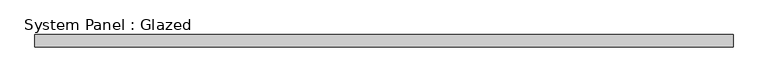
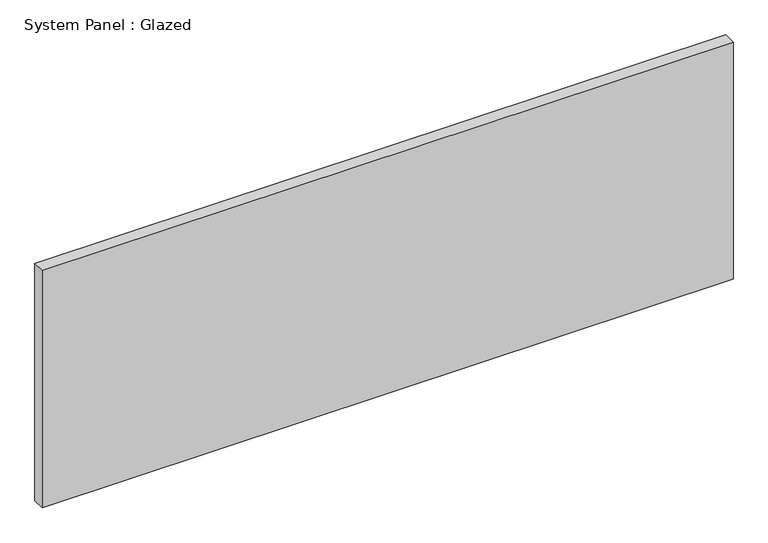
"""IFC4 building model written with IfcOpenShell, lengths in millimetres: plate geometry, System Panel : Glazed."""

from ifc_helpers import new_model, si_unit, origin, origin_with_axes, place, context, project, spatial, polyline, outline, extrude, source, transform, mapped, element, save


def system_panel_glazed_3d3fe78f(model_context):
    return source(origin(), model_context, "Body", "SweptSolid", [
        extrude(outline(polyline([(708.025, 19.05), (-708.025, 19.05), (-708.025, 44.45), (708.025, 44.45), (708.025, 19.05)])), origin_with_axes(), (0.0, 0.0, 1.0), 514.35),
    ])


if __name__ == "__main__":
    model = new_model("IFC4")
    model_context = context("Model", 3, world=origin())
    ifc_project = project(units=[si_unit("LENGTHUNIT", "METRE", prefix="MILLI")], contexts=[model_context])
    site = spatial("IfcSite", under=ifc_project)
    building = spatial("IfcBuilding", under=site)
    placement = place(None, origin())
    system_panel_glazed_shape = system_panel_glazed_3d3fe78f(model_context)
    element("IfcPlate", 1, ObjectType="System Panel : Glazed", at=placement, inside=building, context=model_context, shape_type="MappedRepresentation", body=[
        mapped(system_panel_glazed_shape, transform((0.0, 0.0, 0.0), x_axis=(1.0, 0.0, 0.0), y_axis=(0.0, 1.0, 0.0), z_axis=(0.0, 0.0, 1.0))),
    ])
    save(model, "model.ifc")

# Revit data of these elements
# Type "System Panel : Glazed"
#   Construction Type Id = "GSP4R"
#   Analytic Construction = "1/8 in Pilkington single glazing"
#   Visual Light Transmittance = 0.9
#   Solar Heat Gain Coefficient = 0.86
#   Heat Transfer Coefficient (U) = 1.18115 BTU/(h·ft²·°F)
# Element 1 (IfcPlate, "System Panel : Glazed")
#   Materials on its faces: "Glass"
# Materials
#   "Glass": class "Glass", colour RGB 0 128 192, transparency 0.75, Description = "Soda Lime Glass", Cost = 0
